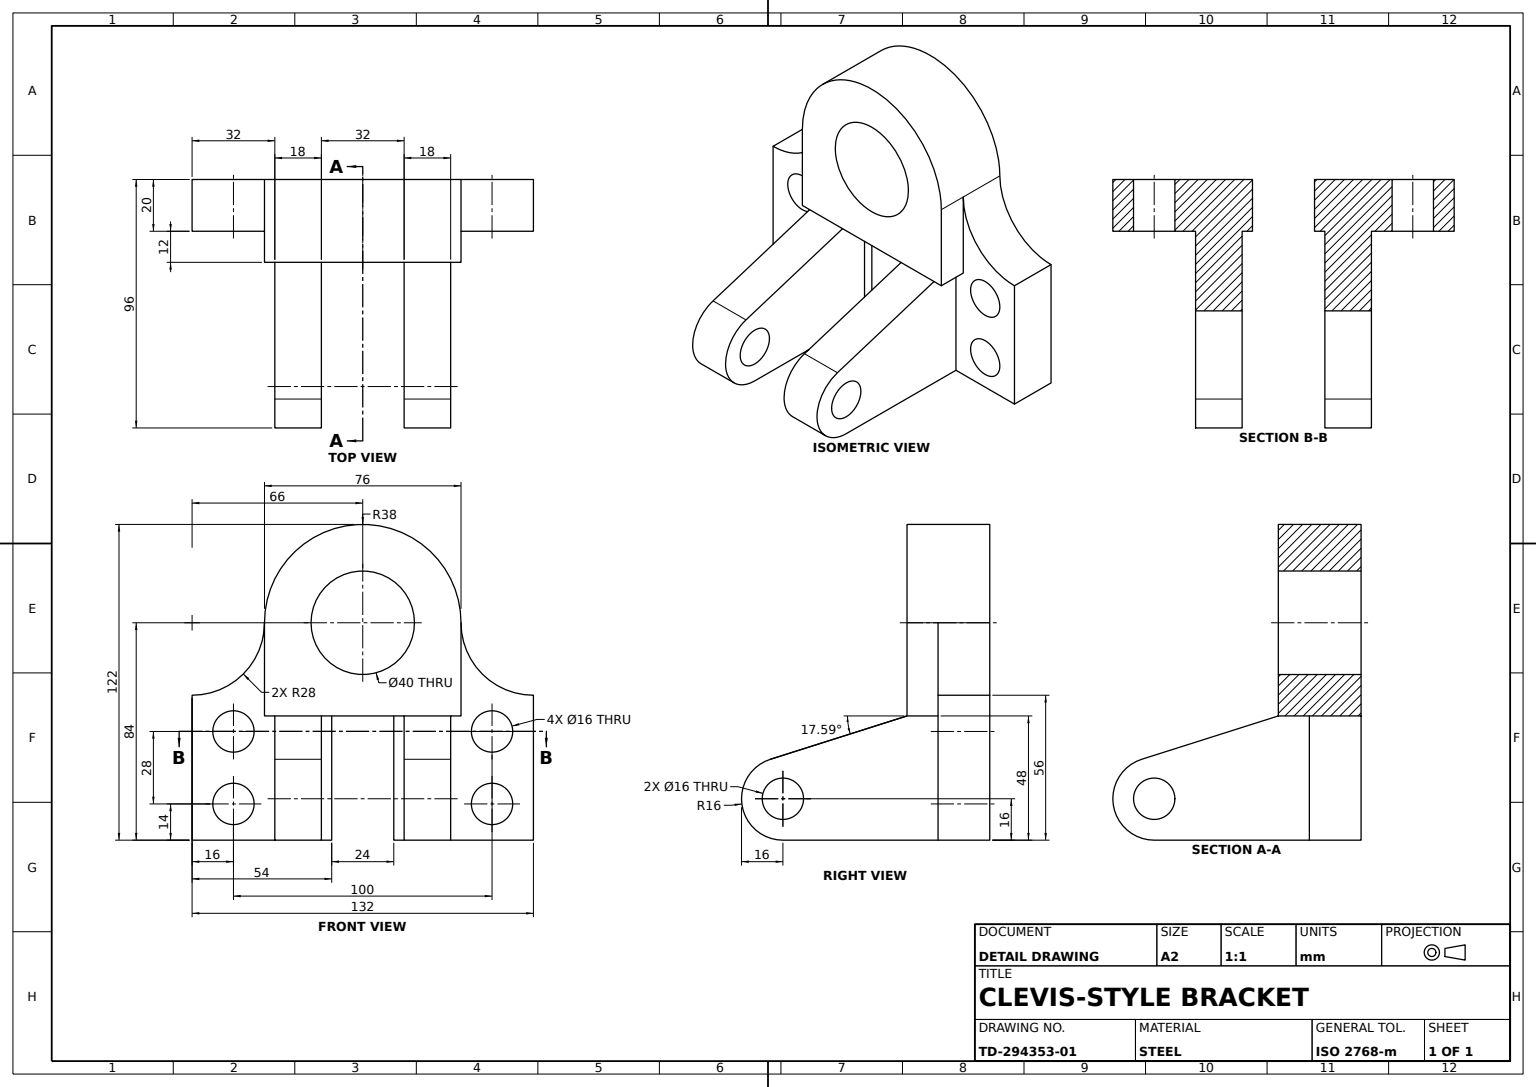
SolidWorks part; units mm, degrees
material "Plain Carbon Steel"
ref_plane "Front Plane" through (0, 0, 0) normal (0, 0, 1) x (1, 0, 0)
ref_plane "Top Plane" through (0, 0, 0) normal (0, 1, 0) x (1, 0, 0)
ref_plane "Right Plane" through (0, 0, 0) normal (1, 0, 0) x (0, 0, -1)
sketch "Base Plate Sketch" plane through (0, 0, 0) normal (0, 0, 1) x (1, 0, 0)
  line L0 (0, 91.8157) -> (0, -97.8862) construction
  line L1 (-66, 61.9187) -> (-66, -22.0813)
  line L4 (-66, -22.0813) -> (-12, -22.0813)
  line L5 (-12, -22.0813) -> (-12, 61.9187)
  line L6 (-66, 61.9187) -> (-12, 61.9187)
  line L7 (66, 61.9187) -> (12, 61.9187)
  line L8 (12, -22.0813) -> (12, 61.9187)
  line L9 (66, -22.0813) -> (12, -22.0813)
  line L10 (66, 61.9187) -> (66, -22.0813)
  circle A1 centre (-50, 19.9187) radius 8
  circle A2 centre (-50, -8.0813) radius 8
  circle A3 centre (50, -8.0813) radius 8
  circle A4 centre (50, 19.9187) radius 8
  dimension "D4" = 12
  dimension "D5" = 16
  dimension "D6" = 16
  dimension "D1" = 84
  dimension "D2" = 54
  dimension "D3" = 84
  dimension "D7" = 28
  dimension "D8" = 16
  dimension "D9" = 14
  dimension "D10" = 61.9187
  dimension "D11" = 19.9187
extrude "Base Plate" add sketch "Base Plate Sketch" against normal blind 20
sketch "Bearing Boss Sketch" plane through (0, 0, -20) normal (0, 0, -1) x (-1, 0, 0)
  line L0 (-66, 61.9187) -> (66, 61.9187) construction
  line L1 (38, 61.9187) -> (38, 25.9187)
  line L2 (38, 25.9187) -> (-38, 25.9187)
  line L3 (-38, 25.9187) -> (-38, 61.9187)
  line L4 (-12, -22.0813) -> (-66, -22.0813) construction
  arc A0 (38, 61.9187) -> (-38, 61.9187) centre (0, 61.9187) ccw
  circle A1 centre (0, 61.9187) radius 20
  dimension "D1" = 76
  dimension "D2" = 40
  dimension "D3" = 48
extrude "Bearing Boss" add sketch "Bearing Boss Sketch" against normal blind 32
sketch "Bore Sketch" plane through (0, 0, 12) normal (0, 0, 1) x (1, 0, 0)
  circle A0 centre (0, 61.9187) radius 20
  dimension "D1" = 40
extrude "Bore Ø40" cut sketch "Bore Sketch" against normal blind 32
sketch "Side Cut Sketch" plane through (0, 0, 0) normal (0, 0, 1) x (1, 0, 0)
  line L0 (-66, 61.9187) -> (-66, -22.0813) construction
  line L1 (0, 120.7966) -> (0, -82.5947) construction
  line L3 (-38, 61.9187) -> (-66, 61.9187)
  line L4 (-66, 61.9187) -> (-66, 33.9187)
  arc A0 (-38, 61.9187) -> (-66, 33.9187) centre (-66, 61.9187) cw
  arc A1 (38, 61.9187) -> (66, 33.9187) centre (66, 61.9187) ccw
  line M6 (-38, 61.9187) -> (-66, 61.9187)
  line M7 (-66, 61.9187) -> (-66, -22.0813)
  dimension "D1" = 56
  dimension "D2" = 28
extrude "Side Cut" cut sketch "Side Cut Sketch" against normal blind 32 contours A0 M6 M7
mirror "Side Cut Mirror" about plane through (0, 0, 0) normal (1, 0, 0) of "Side Cut"
sketch "Clevis Lug Sketch" plane through (0, 0, 0) normal (0, 0, 1) x (1, 0, 0)
  line L0 (-66, -22.0813) -> (-12, -22.0813) construction
  line L1 (-16, -22.0813) -> (-34, -22.0813)
  line L2 (-16, -22.0813) -> (-16, 25.9187)
  line L3 (-16, 25.9187) -> (-34, 25.9187)
  line L4 (-34, -22.0813) -> (-34, 25.9187)
  line L5 (-38, 25.9187) -> (-12, 25.9187) construction
  dimension "D1" = 4
  dimension "D2" = 18
extrude "Clevis Lug" add sketch "Clevis Lug Sketch" along normal blind 76
mirror "Clevis Lug Mirror" about plane through (0, 0, 0) normal (1, 0, 0) of "Clevis Lug"
sketch "Lug End Profile Sketch" plane through (-34, 0, 0) normal (-1, 0, 0) x (0, 0, 1)
  line L0 (76, 25.9187) -> (76, -22.0813) construction
  line L1 (76, -22.0813) -> (0, -22.0813) construction
  line L2 (12, 25.9187) -> (64.8347, 9.1708)
  line L3 (12, 25.9187) -> (76, 25.9187)
  line L4 (76, 25.9187) -> (76, -6.0813)
  line L5 (60, -22.0813) -> (76, -22.0813)
  line L6 (76, -22.0813) -> (76, -6.0813)
  circle A0 centre (60, -6.0813) radius 8
  arc A1 (60, -22.0813) -> (64.8347, 9.1708) centre (60, -6.0813) ccw
  line M2 (0, -22.0813) -> (76, -22.0813)
  line M3 (76, -22.0813) -> (76, 25.9187)
  line M4 (76, 25.9187) -> (12, 25.9187)
  dimension "D1" = 16
  dimension "D3" = 16
  dimension "D2" = 16
  dimension "D4" = 48
extrude "Lug End Profile Cut" cut sketch "Lug End Profile Sketch" against normal blind 76 contours A1 L2 M3 M4 | A1 M2 M3 | A0
